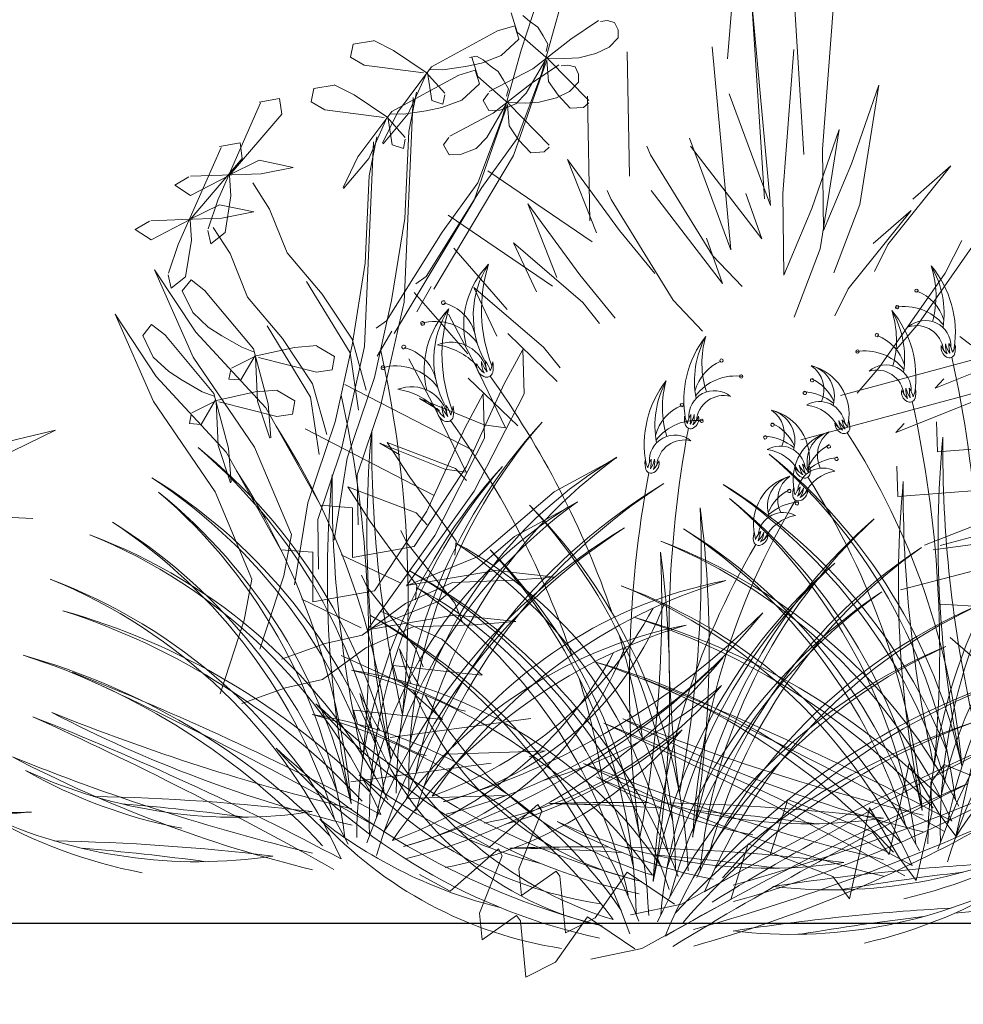
# Model space of a CAD drawing. Units: inches. Extents: x 89 to 490, y -59 to 378.
# Tile 4 of 20: x 300 to 326, y -26 to 1. Entities that reach past the tile are written whole.
import ezdxf

# ---------------------------------------------------------------- set-up
doc = ezdxf.new("R2010")
doc.units = ezdxf.units.IN
doc.header["$MEASUREMENT"] = 0
for name, color, linetype, lineweight in [('A-ANNO-DIMS', 2, 'Continuous', 18), ('L-PLNT', 94, 'Continuous', 18), ('L-PLNT-EDGE', 31, 'Continuous', 25)]:
    doc.layers.add(name, color=color, linetype=linetype, lineweight=lineweight)
doc.layers.add('fl', color=73, linetype='Continuous', lineweight=9, true_color=0xa3d166)
doc.styles.get("Standard").update_dxf_attribs({"font": 'arial.ttf'})
doc.dimstyles.get("Standard").update_dxf_attribs({"dimtxt": 6, "dimasz": 4, "dimexe": 3, "dimexo": 3, "dimgap": 0.09, "dimtad": 0, "dimtih": 1, "dimtoh": 1, "dimdec": 1, "dimzin": 0, "dimdsep": 46, "dimlunit": 3, "dimtxsty": 'Standard', "dimcen": 0.09, "dimadec": 0, "dimazin": 0, "dimtfac": 1, "dimtdec": 1, "dimtofl": 0, "dimtmove": 0, "dimatfit": 3, "dimfxl": 1, "dimtolj": 1, "dimtzin": 0, "dimarcsym": 0})

# ---------------------------------------------------------------- blocks, each defined once
blk = doc.blocks.new('Plantation')
at = {"layer": 'fl'}
for p, q in [((544.751, 40.317), (545.243, 32.557)), ((543.667, 39.099), (544.159, 31.339)), ((543.151, 35.179), (543.425, 38.511)), ((537.49, 35.411), (538.018, 37.033)), ((543.813, 36.723), (544.326, 31.159)), ((537.223, 36.436), (537.387, 35.907)), ((538.054, 34.764), (538.574, 36.629)), ((546.054, 36.651), (545.751, 32.703)), ((537.539, 36.364), (537.724, 36.203)), ((537.724, 36.203), (537.945, 36.043)), ((538.852, 35.714), (539.613, 36.226)), ((539.852, 36.222), (539.671, 36.201)), ((540.053, 36.171), (539.852, 36.222)), ((540.148, 35.972), (540.053, 36.171)), ((535.034, 34.953), (536.847, 35.938)), ((537.317, 36.081), (536.842, 35.939)), ((537.43, 35.711), (537.317, 36.081)), ((537.387, 35.907), (538.239, 35.158)), ((537.945, 36.043), (538.095, 35.809)), ((540.152, 35.754), (540.148, 35.972)), ((533.447, 35.668), (532.891, 35.578)), ((533.453, 35.677), (533.997, 35.404)), ((536.947, 35.264), (537.43, 35.711)), ((537.811, 34.901), (538.852, 35.714)), ((538.095, 35.809), (538.226, 35.574)), ((539.901, 35.494), (540.152, 35.754)), ((532.891, 35.578), (532.818, 35.218)), ((533.997, 35.404), (534.893, 34.802)), ((536.97, 33.546), (537.49, 35.411)), ((538.226, 35.574), (538.175, 35.373)), ((539.54, 35.324), (539.901, 35.494)), ((540.458, 31.956), (540.399, 35.367)), ((542.729, 35.505), (543.242, 29.941)), ((544.97, 35.433), (544.667, 31.485)), ((532.818, 35.218), (533.193, 34.999)), ((536.072, 35.212), (536.272, 35.252)), ((536.14, 35.218), (536.303, 34.689)), ((536.272, 35.252), (536.455, 35.146)), ((536.406, 35.055), (536.947, 35.264)), ((536.455, 35.146), (536.64, 34.985)), ((537.287, 32.524), (538.197, 35.137)), ((537.631, 34.235), (538.179, 35.173)), ((538.197, 35.137), (538.244, 34.555)), ((538.233, 35.192), (538.688, 35.182)), ((538.239, 35.158), (539.347, 34.029)), ((538.688, 35.182), (539.07, 35.207)), ((539.07, 35.207), (539.54, 35.324)), ((533.193, 34.999), (534.817, 34.788)), ((534.104, 33.706), (535.034, 34.953)), ((535.001, 34.884), (535.347, 34.877)), ((535.347, 34.877), (535.969, 34.968)), ((536.234, 34.863), (535.758, 34.721)), ((535.969, 34.968), (536.406, 35.055)), ((536.346, 34.493), (536.234, 34.863)), ((536.616, 34.276), (537.811, 34.901)), ((536.64, 34.985), (536.861, 34.825)), ((536.861, 34.825), (537.011, 34.591)), ((537.768, 34.496), (538.529, 35.008)), ((538.768, 35.004), (538.587, 34.983)), ((538.969, 34.953), (538.768, 35.004)), ((539.064, 34.754), (538.969, 34.953)), ((533.95, 33.735), (535.763, 34.72)), ((534.398, 33.664), (534.897, 34.776)), ((534.893, 34.802), (535.398, 34.236)), ((535.043, 34.034), (534.923, 34.803)), ((536.303, 34.689), (537.155, 33.94)), ((537.011, 34.591), (537.142, 34.356)), ((537.385, 32.991), (538.054, 34.764)), ((538.244, 34.555), (538.505, 34.177)), ((539.068, 34.536), (539.064, 34.754)), ((531.807, 34.36), (531.734, 34)), ((532.363, 34.45), (531.807, 34.36)), ((532.369, 34.459), (532.914, 34.186)), ((535.863, 34.046), (536.346, 34.493)), ((536.727, 33.683), (537.768, 34.496)), ((537.142, 34.356), (537.091, 34.155)), ((538.457, 34.106), (538.817, 34.276)), ((538.817, 34.276), (539.068, 34.536)), ((546.543, 32.293), (547.295, 34.457)), ((547.295, 34.457), (546.775, 31.182)), ((530.309, 33.991), (530.873, 34.089)), ((530.873, 34.089), (530.931, 33.662)), ((532.914, 34.186), (533.809, 33.584)), ((534.528, 34.116), (534.284, 28.508)), ((534.413, 33.182), (534.62, 34.258)), ((535.35, 33.934), (535.043, 34.034)), ((535.322, 33.837), (535.863, 34.046)), ((535.398, 34.187), (535.35, 33.934)), ((536.594, 34.235), (536.452, 34.032)), ((536.452, 34.032), (536.602, 33.762)), ((537.345, 33.938), (537.631, 34.235)), ((537.986, 33.989), (538.457, 34.106)), ((538.505, 34.177), (538.839, 33.819)), ((539.374, 30.738), (539.315, 34.149)), ((544.326, 31.159), (543.192, 34.216)), ((529.72, 32.536), (530.352, 33.967)), ((531.734, 34), (532.109, 33.781)), ((532.109, 33.781), (533.733, 33.57)), ((533.02, 32.488), (533.95, 33.735)), ((534.263, 33.659), (534.885, 33.75)), ((534.885, 33.75), (535.322, 33.837)), ((536.203, 31.306), (537.114, 33.919)), ((536.547, 33.017), (537.095, 33.955)), ((536.602, 33.762), (536.912, 33.767)), ((536.912, 33.767), (537.345, 33.938)), ((537.114, 33.919), (537.16, 33.337)), ((537.149, 33.974), (537.604, 33.964)), ((537.155, 33.94), (538.263, 32.811)), ((537.604, 33.964), (537.986, 33.989)), ((538.839, 33.819), (539.202, 33.843)), ((539.202, 33.843), (539.346, 33.973)), ((530.931, 33.662), (529.502, 31.99)), ((533.315, 32.446), (533.813, 33.558)), ((533.695, 32.866), (534.104, 33.706)), ((533.709, 32.842), (534.398, 33.664)), ((533.809, 33.584), (534.314, 33.018)), ((533.959, 32.816), (533.839, 33.585)), ((533.917, 33.666), (534.263, 33.659)), ((535.533, 33.058), (536.727, 33.683)), ((536.301, 31.773), (536.97, 33.546)), ((537.16, 33.337), (537.421, 32.959)), ((545.459, 31.075), (546.211, 33.239)), ((546.211, 33.239), (545.691, 29.964)), ((533.33, 31.964), (533.536, 33.04)), ((534.315, 32.969), (534.266, 32.716)), ((534.3, 30.796), (534.413, 33.182)), ((535.51, 33.017), (535.368, 32.814)), ((536.261, 32.72), (536.547, 33.017)), ((536.41, 31.646), (537.385, 32.991)), ((537.421, 32.959), (537.755, 32.601)), ((543.242, 29.941), (542.108, 32.998)), ((528.636, 31.318), (529.268, 32.749)), ((529.225, 32.773), (529.789, 32.871)), ((529.789, 32.871), (529.847, 32.444)), ((533.444, 32.898), (533.2, 27.29)), ((534.266, 32.716), (533.959, 32.816)), ((535.368, 32.814), (535.518, 32.544)), ((535.828, 32.549), (536.261, 32.72)), ((538.119, 32.625), (538.262, 32.755)), ((540.935, 32.782), (541.041, 32.543)), ((542.136, 32.784), (544.093, 30.239)), ((545.751, 32.703), (545.778, 30.468)), ((529.847, 32.444), (528.418, 30.772)), ((529.179, 31.302), (529.72, 32.536)), ((530.312, 32.394), (529.465, 31.976)), ((531.245, 32.196), (530.312, 32.394)), ((532.611, 31.648), (533.02, 32.488)), ((532.625, 31.624), (533.315, 32.446)), ((535.097, 28.864), (537.287, 32.524)), ((535.518, 32.544), (535.828, 32.549)), ((537.755, 32.601), (538.119, 32.625)), ((539.558, 30.402), (538.76, 32.416)), ((538.76, 32.416), (540.188, 30.472)), ((541.041, 32.543), (542.739, 29.781)), ((530.369, 32.023), (531.239, 32.198)), ((545.778, 30.468), (546.543, 32.293)), ((549.267, 32.24), (547.541, 30.09)), ((548.228, 31.329), (549.267, 32.24)), ((528.385, 31.945), (527.999, 31.712)), ((528.427, 31.957), (529.301, 31.987)), ((528.431, 31.43), (529.49, 31.977)), ((529.301, 31.987), (530.369, 32.023)), ((529.537, 31.424), (529.502, 31.977)), ((533.216, 29.578), (533.33, 31.964)), ((539.439, 30.158), (536.579, 32.105)), ((527.999, 31.712), (528.431, 31.43)), ((530.135, 31.772), (530.597, 31.058)), ((534.889, 29.212), (536.41, 31.646)), ((535.326, 30.428), (536.301, 31.773)), ((528.095, 30.084), (528.636, 31.318)), ((529.379, 30.415), (529.537, 31.424)), ((534.013, 27.646), (536.203, 31.306)), ((539.852, 31.564), (539.957, 31.324)), ((539.957, 31.324), (541.655, 28.563)), ((541.053, 31.566), (543.009, 29.021)), ((544.093, 30.239), (543.655, 31.48)), ((544.667, 31.485), (544.695, 29.25)), ((529.228, 31.176), (528.381, 30.758)), ((528.914, 30.515), (529.179, 31.302)), ((530.161, 30.978), (529.228, 31.176)), ((530.597, 31.058), (531.075, 29.859)), ((538.474, 29.184), (537.677, 31.198)), ((537.677, 31.198), (539.104, 29.254)), ((544.695, 29.25), (545.459, 31.075)), ((546.775, 31.182), (546.061, 29.311)), ((527.343, 30.739), (528.217, 30.769)), ((528.217, 30.769), (529.286, 30.805)), ((529.286, 30.805), (530.155, 30.98)), ((533.94, 28.547), (534.3, 30.796)), ((538.355, 28.94), (535.495, 30.887)), ((548.183, 31.022), (546.458, 28.872)), ((547.144, 30.111), (548.183, 31.022)), ((527.301, 30.727), (526.915, 30.494)), ((527.348, 30.212), (528.406, 30.759)), ((528.453, 30.206), (528.419, 30.759)), ((529.051, 30.554), (529.513, 29.84)), ((550.2, 30.521), (548.393, 27.932)), ((526.915, 30.494), (527.348, 30.212)), ((528.901, 30.47), (528.982, 30.107)), ((528.982, 30.107), (529.379, 30.415)), ((533.805, 27.994), (535.326, 30.428)), ((540.188, 30.472), (541.152, 29.289)), ((543.009, 29.021), (542.572, 30.262)), ((527.83, 29.297), (528.095, 30.084)), ((528.295, 29.197), (528.453, 30.206)), ((535.646, 29.986), (537.112, 28.305)), ((537.912, 28.79), (537.283, 30.13)), ((537.283, 30.13), (539.186, 28.493)), ((545.691, 29.964), (544.977, 28.093)), ((547.541, 30.09), (547.178, 29.349)), ((549.572, 30.194), (549.117, 29.303)), ((529.513, 29.84), (529.991, 28.641)), ((531.075, 29.859), (532.038, 28.726)), ((542.739, 29.781), (543.546, 28.933)), ((532.856, 27.329), (533.216, 29.578)), ((528.499, 27.001), (527.445, 29.395)), ((527.445, 29.395), (528.573, 27.684)), ((527.817, 29.252), (527.898, 28.889)), ((527.898, 28.889), (528.295, 29.197)), ((534.604, 29.008), (534.889, 29.212)), ((539.104, 29.254), (540.068, 28.071)), ((549.117, 29.303), (547.309, 26.714)), ((528.205, 28.812), (528.446, 29.115)), ((528.446, 29.115), (528.836, 28.808)), ((531.611, 29.076), (532.806, 27.116)), ((534.63, 28.241), (535.028, 28.931)), ((536.828, 27.572), (536.199, 28.912)), ((536.199, 28.912), (538.102, 27.275)), ((528.49, 28.219), (528.205, 28.812)), ((530.154, 27.225), (528.831, 28.809)), ((529.991, 28.641), (530.954, 27.508)), ((532.038, 28.726), (532.857, 27.49)), ((534.563, 28.768), (536.028, 27.087)), ((546.458, 28.872), (546.094, 28.131)), ((533.477, 26.441), (533.94, 28.547)), ((534.284, 28.508), (533.65, 25.695)), ((539.186, 28.493), (539.643, 27.925)), ((541.655, 28.563), (542.462, 27.715)), ((527.415, 25.783), (526.361, 28.177)), ((526.361, 28.177), (527.489, 26.466)), ((528.916, 27.825), (528.49, 28.219)), ((536.23, 26.788), (535.502, 28.173)), ((527.121, 27.594), (527.363, 27.897)), ((527.363, 27.897), (527.753, 27.59)), ((529.289, 27.583), (528.916, 27.825)), ((530.527, 27.858), (531.722, 25.898)), ((533.521, 27.79), (533.805, 27.994)), ((548.393, 27.932), (547.785, 27.231)), ((527.406, 27.001), (527.121, 27.594)), ((529.07, 26.007), (527.747, 27.591)), ((528.573, 27.684), (530.491, 25.61)), ((529.835, 27.269), (529.289, 27.583)), ((533.546, 27.023), (533.944, 27.713)), ((537.124, 27.645), (538.482, 26.33)), ((552.203, 27.553), (546.246, 25.952)), ((548.842, 26.149), (552.295, 27.53)), ((549.516, 27.567), (549.816, 27.334)), ((530.158, 27.149), (529.835, 27.269)), ((531.283, 27.262), (530.229, 27.033)), ((530.954, 27.508), (531.774, 26.272)), ((531.889, 27.315), (531.283, 27.262)), ((531.892, 27.304), (532.376, 27.016)), ((532.393, 25.223), (532.856, 27.329)), ((533.2, 27.29), (532.566, 24.477)), ((532.857, 27.49), (533.245, 26.093)), ((538.102, 27.275), (538.559, 26.707)), ((527.832, 26.607), (527.406, 27.001)), ((530.187, 24.53), (528.499, 27.001)), ((530.229, 27.033), (529.55, 26.693)), ((529.807, 26.374), (530.201, 27.045)), ((530.558, 25.723), (530.154, 27.225)), ((530.269, 25.793), (530.215, 27.01)), ((531.881, 26.589), (530.294, 26.991)), ((532.376, 27.016), (532.311, 26.654)), ((532.806, 27.116), (533.038, 25.548)), ((537.031, 26.271), (537.534, 27.212)), ((537.534, 27.212), (537.575, 25.998)), ((535.146, 25.57), (534.418, 26.955)), ((537.067, 25.066), (536.23, 26.788)), ((527.489, 26.466), (529.407, 24.392)), ((528.205, 26.365), (527.832, 26.607)), ((529.532, 26.647), (529.484, 26.394)), ((532.311, 26.654), (531.881, 26.589)), ((547.309, 26.714), (546.701, 26.013)), ((528.751, 26.051), (528.205, 26.365)), ((529.484, 26.394), (529.807, 26.374)), ((531.774, 26.272), (532.162, 24.875)), ((536.192, 24.428), (532.66, 26.252)), ((532.726, 24.228), (533.477, 26.441)), ((535.99, 23.999), (537.031, 26.271)), ((536.041, 26.427), (537.398, 25.112)), ((551.119, 26.335), (545.162, 24.734)), ((547.759, 24.931), (551.212, 26.312)), ((549.077, 26.4), (548.842, 26.149)), ((529.074, 25.931), (528.751, 26.051)), ((529.474, 24.505), (529.07, 26.007)), ((530.199, 26.044), (529.145, 25.815)), ((530.806, 26.097), (530.199, 26.044)), ((530.808, 26.086), (531.292, 25.798)), ((535.947, 25.053), (536.45, 25.994)), ((537.575, 25.998), (536.208, 23.326)), ((536.45, 25.994), (536.491, 24.78)), ((529.104, 23.312), (527.415, 25.783)), ((529.145, 25.815), (528.466, 25.475)), ((528.723, 25.156), (529.117, 25.827)), ((529.185, 24.575), (529.132, 25.792)), ((530.797, 25.371), (529.21, 25.773)), ((530.607, 24.774), (530.269, 25.793)), ((530.628, 24.791), (530.558, 25.723)), ((531.292, 25.798), (531.227, 25.436)), ((531.722, 25.898), (531.954, 24.33)), ((533.65, 25.695), (533.001, 23.77)), ((535.252, 25.539), (534.706, 25.861)), ((534.706, 25.861), (536.481, 25.144)), ((528.448, 25.429), (528.4, 25.176)), ((530.491, 25.61), (531.992, 22.939)), ((531.227, 25.436), (530.797, 25.371)), ((535.983, 23.848), (535.146, 25.57)), ((528.4, 25.176), (528.723, 25.156)), ((531.642, 23.01), (532.393, 25.223)), ((536.481, 25.144), (537.067, 25.066)), ((547.993, 25.182), (547.759, 24.931)), ((548.874, 25.226), (548.902, 24.401)), ((524.733, 24.997), (522.589, 23.962)), ((523.242, 24.639), (524.733, 24.997)), ((535.108, 23.21), (531.576, 25.034)), ((534.907, 22.781), (535.947, 25.053)), ((529.523, 23.556), (529.185, 24.575)), ((534.168, 24.321), (533.622, 24.643)), ((533.622, 24.643), (535.397, 23.926)), ((534.439, 23.713), (533.823, 24.664)), ((533.823, 24.664), (535.695, 23.95)), ((536.491, 24.78), (535.124, 22.108)), ((548.902, 24.401), (552.345, 24.664)), ((529.407, 24.392), (530.908, 21.721)), ((529.544, 23.573), (529.474, 24.505)), ((531.193, 22.134), (530.187, 24.53)), ((532.566, 24.477), (531.917, 22.552)), ((532.365, 21.98), (532.726, 24.228)), ((538.396, 23.303), (540.114, 24.237)), ((533.001, 23.77), (533.025, 22.404)), ((534.558, 21.811), (535.99, 23.999)), ((535.397, 23.926), (535.983, 23.848)), ((535.695, 23.95), (535.998, 23.62)), ((547.79, 24.008), (547.818, 23.183)), ((535.714, 21.958), (534.439, 23.713)), ((530.109, 20.916), (529.104, 23.312)), ((533.355, 22.495), (532.739, 23.446)), ((532.739, 23.446), (534.611, 22.732)), ((536.208, 23.326), (534.352, 20.735)), ((536.318, 21.531), (538.396, 23.303)), ((547.818, 23.183), (551.261, 23.446)), ((531.281, 20.762), (531.642, 23.01)), ((531.992, 22.939), (532.869, 22.872)), ((537.312, 22.085), (539.031, 23.019)), ((520.615, 22.763), (524.11, 22.574)), ((532.869, 22.872), (532.867, 21.511)), ((533.474, 20.593), (534.907, 22.781)), ((534.611, 22.732), (534.914, 22.402)), ((550.991, 22.805), (548.544, 21.846)), ((531.917, 22.552), (531.941, 21.186)), ((534.63, 20.74), (533.355, 22.495)), ((552.039, 22.642), (548.978, 21.84)), ((530.988, 21.009), (531.193, 22.134)), ((534.355, 21.911), (534.197, 22.246)), ((535.124, 22.108), (533.268, 19.517)), ((535.675, 20.255), (534.355, 21.911)), ((535.234, 20.313), (537.312, 22.085)), ((535.679, 21.568), (535.714, 21.958)), ((548.789, 21.719), (551.609, 22.101)), ((530.908, 21.721), (531.785, 21.654)), ((531.785, 21.654), (531.783, 20.293)), ((532.867, 21.511), (534.558, 21.811)), ((532.562, 21.58), (534.191, 20.801)), ((534.352, 20.735), (536.318, 21.531)), ((550.955, 21.424), (547.894, 20.622)), ((536.74, 21.145), (534.353, 20.74)), ((536.719, 21.156), (538.427, 20.971)), ((529.904, 19.791), (530.109, 20.916)), ((530.328, 18.993), (530.988, 21.009)), ((533.271, 20.693), (533.113, 21.028)), ((535.613, 20.826), (534.32, 20.248)), ((537.263, 20.883), (535.613, 20.826)), ((538.427, 20.971), (537.263, 20.883)), ((531.783, 20.293), (533.474, 20.593)), ((534.591, 19.037), (533.271, 20.693)), ((534.595, 20.35), (534.63, 20.74)), ((531.478, 20.362), (533.107, 19.583)), ((534.32, 20.248), (533.134, 19.381)), ((533.268, 19.517), (535.234, 20.313)), ((535.887, 19.727), (535.675, 20.255)), ((535.32, 19.271), (533.641, 20.04)), ((548.981, 20.225), (552.476, 20.037)), ((529.244, 17.775), (529.904, 19.791)), ((535.657, 19.927), (533.269, 19.522)), ((535.636, 19.938), (537.343, 19.753)), ((537.343, 19.753), (536.18, 19.665)), ((534.529, 19.608), (533.236, 19.03)), ((536.18, 19.665), (534.529, 19.608)), ((533.134, 19.381), (532.121, 19.152)), ((536.423, 18.287), (535.32, 19.271)), ((549.247, 19.315), (551.779, 17.113)), ((532.121, 19.152), (530.92, 18.722)), ((533.236, 19.03), (532.05, 18.163)), ((534.804, 18.509), (534.591, 19.037)), ((534.236, 18.053), (532.557, 18.822)), ((534.094, 18.159), (533.983, 18.544)), ((533.983, 18.544), (535.691, 18.36)), ((535.691, 18.36), (536.423, 18.287)), ((532.05, 18.163), (531.037, 17.934)), ((535.774, 17.342), (534.094, 18.159)), ((531.037, 17.934), (529.836, 17.504)), ((535.339, 17.069), (534.236, 18.053)), ((533.01, 16.941), (532.899, 17.326)), ((532.899, 17.326), (534.607, 17.142)), ((535.97, 17.3), (535.774, 17.342)), ((533.906, 16.575), (537.756, 17.091)), ((534.607, 17.142), (535.339, 17.069)), ((534.69, 16.124), (533.01, 16.941)), ((538.146, 16.207), (537.175, 16.174)), ((537.714, 16.047), (538.146, 16.207)), ((534.886, 16.082), (534.69, 16.124)), ((537.175, 16.174), (535.476, 16.116)), ((532.822, 15.357), (536.672, 15.873)), ((548.124, 15.867), (547.577, 13.369)), ((548.949, 14.485), (548.124, 15.867)), ((549.09, 15.837), (548.718, 15.338)), ((550.076, 15.433), (549.09, 15.837)), ((549.83, 15.731), (549.407, 13.869)), ((548.718, 15.338), (548.746, 14.513)), ((536.091, 14.956), (534.392, 14.898)), ((537.063, 14.989), (536.091, 14.956)), ((536.631, 14.829), (537.063, 14.989)), ((544.803, 14.879), (544.32, 13.355)), ((547.118, 13.985), (544.803, 14.879)), ((537.953, 14.742), (536.632, 13.579)), ((538.057, 14.551), (537.953, 14.742)), ((547.04, 14.649), (546.493, 12.151)), ((547.865, 13.267), (547.04, 14.649)), ((537.43, 12.974), (538.057, 14.551)), ((548.746, 14.513), (548.323, 12.651)), ((549.407, 13.869), (548.949, 14.485)), ((536.632, 13.579), (535.79, 14.036)), ((547.577, 13.369), (547.118, 13.985)), ((536.869, 13.524), (535.548, 12.361)), ((536.973, 13.333), (536.869, 13.524)), ((543.719, 13.661), (543.236, 12.137)), ((546.034, 12.767), (543.719, 13.661)), ((536.346, 11.756), (536.973, 13.333)), ((544.32, 13.355), (541.887, 12.008)), ((548.323, 12.651), (547.865, 13.267)), ((537.504, 12.248), (537.43, 12.974)), ((535.548, 12.361), (534.706, 12.818)), ((538.453, 12.912), (537.504, 12.248)), ((538.555, 12.77), (538.453, 12.912)), ((538.705, 11.219), (538.555, 12.77)), ((540.399, 12.881), (539.518, 11.636)), ((541.693, 12.002), (540.399, 12.881)), ((546.493, 12.151), (546.034, 12.767)), ((541.887, 12.008), (540.487, 11.717)), ((543.236, 12.137), (540.803, 10.79)), ((536.42, 11.03), (536.346, 11.756)), ((537.369, 11.694), (536.42, 11.03)), ((537.471, 11.552), (537.369, 11.694)), ((539.315, 11.663), (538.434, 10.418)), ((539.518, 11.636), (538.705, 11.219)), ((540.609, 10.784), (539.315, 11.663)), ((537.622, 10.001), (537.471, 11.552)), ((540.803, 10.79), (539.403, 10.499)), ((538.434, 10.418), (537.622, 10.001))]:
    blk.add_line(p, q, dxfattribs=at)
for centre, radius, start, end in [((538.293, 27.882), 2.375, 135.5632, 193.7293), ((538.781, 28.132), 2.601, 147.096, 209.2874), ((540.633, 28.287), 4.227, 162.6858, 201.1197), ((546.541, 27.672), 2.854, 351.4134, 39.8275), ((546.256, 28.682), 2.608, 344.3064, 18.279), ((546.485, 28.192), 2.6, 351.5096, 30.1949), ((548.325, 28.821), 0.0459, 7.5892, 187.5892), ((548.325, 28.821), 0.0459, 187.5892, 7.5892), ((547.89, 27.65), 1.243, 16.8512, 68.8014), ((535.359, 28.494), 0.053, 11.802, 191.802), ((535.359, 28.494), 0.053, 191.802, 11.802), ((535.098, 27.351), 1.163, 13.7128, 76.1437), ((547.799, 28.369), 0.0459, 7.5892, 187.5892), ((547.997, 27.001), 1.386, 39.5069, 100.1323), ((547.799, 28.369), 0.0459, 187.5892, 7.5892), ((537.21, 26.664), 2.375, 135.5632, 193.7293), ((537.697, 26.914), 2.601, 147.096, 209.2874), ((539.549, 27.069), 4.227, 162.6858, 201.1197), ((545.457, 26.454), 2.854, 351.4134, 39.8275), ((545.172, 27.464), 2.608, 344.3064, 18.279), ((545.401, 26.974), 2.6, 351.5096, 30.1949), ((534.791, 27.927), 0.053, 11.802, 191.802), ((535.138, 26.561), 1.416, 35.6636, 106.404), ((534.791, 27.927), 0.053, 191.802, 11.802), ((548.57, 27.303), 0.701, 357.4175, 130.8703), ((548.32, 27.109), 0.754, 6.9832, 106.1055), ((544.805, 25.819), 2.854, 142.1725, 190.5866), ((544.843, 26.34), 2.6, 151.8051, 190.4904), ((545.055, 26.838), 2.608, 163.721, 197.6936), ((547.241, 27.603), 0.0459, 7.5892, 187.5892), ((547.241, 27.603), 0.0459, 187.5892, 7.5892), ((546.806, 26.432), 1.243, 16.8512, 68.8014), ((534.275, 27.276), 0.053, 11.802, 191.802), ((534.275, 27.276), 0.053, 191.802, 11.802), ((534.014, 26.132), 1.163, 13.7128, 76.1437), ((535.571, 26.397), 1.01, 11.1862, 111.7493), ((534.913, 25.471), 1.886, 44.0209, 81.3627), ((549.289, 27.258), 0.289, 168.1654, 242.3938), ((549.56, 27.536), 0.596, 201.5294, 228.9216), ((549.687, 27.312), 0.565, 174.5103, 203.5444), ((549.838, 27.532), 0.733, 193.0983, 215.538), ((550.524, 27.366), 1.308, 179.8013, 191.4565), ((548.639, 26.985), 0.694, 12.1333, 33.7421), ((548.367, 27.577), 1.049, 334.86, 346.6738), ((548.799, 27.25), 0.595, 343.9406, 8.2206), ((502.903, 20.338), 31.492, 354.2791, 12.5427), ((546.715, 27.151), 0.0459, 7.5892, 187.5892), ((546.914, 25.783), 1.386, 39.5069, 100.1323), ((546.715, 27.151), 0.0459, 187.5892, 7.5892), ((549.228, 27.134), 0.151, 241.146, 341.1111), ((518.556, 20.16), 31.492, 354.2791, 12.5427), ((533.707, 26.709), 0.053, 11.802, 191.802), ((534.055, 25.343), 1.416, 35.6636, 106.404), ((533.707, 26.709), 0.053, 191.802, 11.802), ((536.603, 26.772), 0.334, 172.3781, 246.6066), ((536.893, 27.116), 0.689, 205.7422, 233.1344), ((537.058, 26.869), 0.654, 178.723, 207.7572), ((537.214, 27.135), 0.848, 197.3111, 219.7508), ((535.876, 26.402), 0.803, 16.3461, 37.9549), ((538.019, 27.002), 1.513, 184.0141, 195.6693), ((535.514, 27.061), 1.213, 339.0728, 350.8866), ((536.04, 26.721), 0.688, 348.1534, 12.4334), ((543.458, 25.75), 1.243, 113.1986, 165.1488), ((542.982, 26.905), 0.0459, 354.4108, 174.4108), ((542.982, 26.905), 0.0459, 174.4108, 354.4108), ((545.216, 25.932), 0.863, 342.816, 75.0201), ((544.998, 26.106), 0.793, 335.7976, 56.2278), ((545.111, 25.437), 1.368, 349.633, 76.1366), ((547.486, 26.085), 0.701, 357.4175, 130.8703), ((536.544, 26.624), 0.175, 245.3588, 345.3239), ((516.603, 12.04), 24.696, 18.7875, 35.7756), ((543.373, 25.098), 1.386, 81.8677, 142.4931), ((543.523, 26.471), 0.0459, 354.4108, 174.4108), ((543.523, 26.471), 0.0459, 174.4108, 354.4108), ((547.237, 25.891), 0.754, 6.9832, 106.1055), ((534.487, 25.179), 1.01, 11.1862, 111.7493), ((543.721, 24.601), 2.854, 142.1725, 190.5866), ((543.759, 25.122), 2.6, 151.8051, 190.4904), ((543.971, 25.62), 2.608, 163.721, 197.6936), ((545.466, 26.365), 0.0459, 19.649, 199.649), ((545.466, 26.365), 0.0459, 199.649, 19.649), ((544.931, 25.279), 1.243, 24.0842, 65.3008), ((501.819, 19.12), 31.492, 354.2791, 12.5427), ((533.829, 24.253), 1.886, 44.0209, 81.3627), ((542.79, 25.379), 0.701, 51.1297, 184.5825), ((543.046, 25.194), 0.754, 75.8945, 175.0168), ((545.267, 26.018), 0.0459, 19.649, 199.649), ((545.267, 26.018), 0.0459, 199.649, 19.649), ((545.172, 24.667), 1.386, 50.416, 87.3549), ((548.205, 26.04), 0.289, 168.1654, 242.3938), ((548.477, 26.318), 0.596, 201.5294, 228.9216), ((548.603, 26.094), 0.565, 174.5103, 203.5444), ((548.754, 26.314), 0.733, 193.0983, 215.538), ((549.44, 26.148), 1.308, 179.8013, 191.4565), ((547.555, 25.767), 0.694, 12.1333, 33.7421), ((547.284, 26.359), 1.049, 334.86, 346.6738), ((547.716, 26.032), 0.595, 343.9406, 8.2206), ((535.974, 25.65), 0.654, 178.723, 207.7572), ((536.13, 25.917), 0.848, 197.3111, 219.7508), ((534.793, 25.184), 0.803, 16.3461, 37.9549), ((536.935, 25.784), 1.513, 184.0141, 195.6693), ((534.43, 25.843), 1.213, 339.0728, 350.8866), ((534.956, 25.503), 0.688, 348.1534, 12.4334), ((542.374, 24.532), 1.243, 113.1986, 165.1488), ((541.898, 25.687), 0.0459, 354.4108, 174.4108), ((541.898, 25.687), 0.0459, 174.4108, 354.4108), ((545.674, 25.086), 0.696, 9.2042, 120.225), ((545.159, 24.545), 1.154, 27.9293, 81.8071), ((548.144, 25.916), 0.151, 241.146, 341.1111), ((517.472, 18.942), 31.492, 354.2791, 12.5427), ((535.52, 25.554), 0.334, 172.3781, 246.6066), ((535.809, 25.898), 0.689, 205.7422, 233.1344), ((542.563, 25.318), 0.595, 173.7794, 198.0594), ((542.983, 25.66), 1.049, 195.3262, 207.14), ((542.733, 25.059), 0.694, 148.2579, 169.8667), ((540.835, 25.374), 1.308, 350.5435, 2.1987), ((541.515, 25.564), 0.733, 326.462, 348.9017), ((541.674, 25.349), 0.565, 338.4556, 7.4897), ((541.792, 25.577), 0.596, 313.0784, 340.4706), ((542.073, 25.309), 0.289, 299.6062, 13.8346), ((544.132, 24.714), 0.863, 342.816, 75.0201), ((543.914, 24.888), 0.793, 335.7976, 56.2278), ((544.027, 24.219), 1.368, 349.633, 76.1366), ((513.782, 14.158), 20.216, 5.151, 32.7872), ((549.271, 14.948), 15.201, 137.4916, 179.6099), ((549.333, 15.438), 14.921, 139.0392, 181.297), ((535.46, 25.406), 0.175, 245.3588, 345.3239), ((515.52, 10.822), 24.696, 18.7875, 35.7756), ((542.289, 23.88), 1.386, 81.8677, 142.4931), ((542.138, 25.187), 0.151, 200.8889, 300.854), ((542.439, 25.253), 0.0459, 174.4108, 354.4108), ((542.439, 25.253), 0.0459, 354.4108, 174.4108), ((544.382, 25.147), 0.0459, 19.649, 199.649), ((544.382, 25.147), 0.0459, 199.649, 19.649), ((543.847, 24.061), 1.243, 24.0842, 65.3008), ((546.381, 25.187), 0.289, 180.2252, 254.4537), ((546.589, 25.516), 0.596, 213.5892, 240.9815), ((546.759, 25.324), 0.565, 186.5701, 215.6042), ((546.861, 25.571), 0.733, 205.1582, 227.5978), ((545.802, 24.785), 0.694, 24.1932, 45.802), ((547.567, 25.551), 1.308, 191.8611, 203.5164), ((545.414, 25.307), 1.049, 346.9198, 358.7337), ((545.904, 25.077), 0.595, 356.0005, 20.2804), ((563.159, 22.183), 29.894, 174.6174, 191.9895), ((567.384, 24.718), 33.989, 179.5471, 192.7817), ((541.706, 24.161), 0.701, 51.1297, 184.5825), ((573.035, 19.288), 31.492, 169.4573, 187.7209), ((544.183, 24.8), 0.0459, 19.649, 199.649), ((544.088, 23.449), 1.386, 50.416, 87.3549), ((546.312, 23.635), 1.368, 105.8634, 192.367), ((546.19, 24.126), 0.863, 106.9799, 199.184), ((546.402, 24.308), 0.793, 125.7722, 206.2024), ((546.348, 25.054), 0.151, 253.2058, 353.1709), ((529.435, 13.979), 20.216, 5.151, 32.7872), ((541.962, 23.976), 0.754, 75.8945, 175.0168), ((544.183, 24.8), 0.0459, 199.649, 19.649), ((544.59, 23.867), 0.696, 9.2042, 120.225), ((546.497, 23.483), 1.243, 116.6992, 157.9158), ((545.925, 24.55), 0.0459, 162.351, 342.351), ((545.925, 24.55), 0.0459, 342.351, 162.351), ((578.812, 22.005), 29.894, 174.6174, 191.9895), ((583.037, 24.54), 33.989, 179.5471, 192.7817), ((518.937, 13.181), 14.921, 7.1968, 49.4547), ((519.071, 12.705), 15.201, 12.4122, 51.0023), ((544.075, 23.327), 1.154, 27.9293, 81.8071), ((534.591, 13.003), 14.921, 7.1968, 49.4547), ((534.724, 12.527), 15.201, 12.4122, 51.0023), ((546.191, 13.886), 12.017, 120.3536, 167.8423), ((548.22, 13.014), 13.856, 125.7805, 169.1581), ((541.479, 24.1), 0.595, 173.7794, 198.0594), ((541.899, 24.442), 1.049, 195.3262, 207.14), ((541.649, 23.841), 0.694, 148.2579, 169.8667), ((539.751, 24.156), 1.308, 350.5435, 2.1987), ((540.431, 24.346), 0.733, 326.462, 348.9017), ((540.59, 24.131), 0.565, 338.4556, 7.4897), ((540.708, 24.359), 0.596, 313.0784, 340.4706), ((540.989, 24.091), 0.289, 299.6062, 13.8346), ((545.675, 24.106), 0.565, 186.5701, 215.6042), ((545.778, 24.353), 0.733, 205.1582, 227.5978), ((544.719, 23.567), 0.694, 24.1932, 45.802), ((546.483, 24.333), 1.308, 191.8611, 203.5164), ((544.33, 24.089), 1.049, 346.9198, 358.7337), ((546.278, 22.863), 1.386, 94.6451, 131.584), ((544.821, 23.859), 0.595, 356.0005, 20.2804), ((546.136, 24.21), 0.0459, 162.351, 342.351), ((546.136, 24.21), 0.0459, 342.351, 162.351), ((512.698, 12.94), 20.216, 5.151, 32.7872), ((562.075, 20.965), 29.894, 174.6174, 191.9895), ((566.3, 23.5), 33.989, 179.5471, 192.7817), ((548.187, 13.73), 15.201, 137.4916, 179.6099), ((548.249, 14.22), 14.921, 139.0392, 181.297), ((571.951, 18.07), 31.492, 169.4573, 187.7209), ((541.055, 23.969), 0.151, 200.8889, 300.854), ((545.298, 23.969), 0.289, 180.2252, 254.4537), ((545.505, 24.298), 0.596, 213.5892, 240.9815), ((545.762, 23.264), 0.696, 61.775, 172.7958), ((545.264, 23.836), 0.151, 253.2058, 353.1709), ((546.296, 22.742), 1.154, 100.1929, 154.0707), ((563.84, 13.552), 15.201, 137.4916, 179.6099), ((563.902, 14.042), 14.921, 139.0392, 181.297), ((519.189, 11.215), 14.921, 16.8321, 56.7339), ((519.381, 10.76), 15.201, 21.5651, 58.2814), ((550.014, 9.293), 16.642, 121.1471, 160.292), ((550.148, 9.85), 16.239, 122.567, 163.1344), ((534.842, 11.037), 14.921, 16.8321, 56.7339), ((535.034, 10.582), 15.201, 21.5651, 58.2814), ((545.228, 22.417), 1.368, 105.8634, 192.367), ((545.107, 22.908), 0.863, 106.9799, 199.184), ((545.318, 23.09), 0.793, 125.7722, 206.2024), ((528.351, 12.761), 20.216, 5.151, 32.7872), ((577.728, 20.787), 29.894, 174.6174, 191.9895), ((581.953, 23.322), 33.989, 179.5471, 192.7817), ((517.854, 11.963), 14.921, 7.1968, 49.4547), ((517.987, 11.487), 15.201, 12.4122, 51.0023), ((545.413, 22.265), 1.243, 116.6992, 157.9158), ((544.841, 23.332), 0.0459, 162.351, 342.351), ((544.841, 23.332), 0.0459, 342.351, 162.351), ((545.532, 23.248), 0.595, 161.7196, 185.9995), ((546.014, 23.494), 1.049, 183.2663, 195.0802), ((545.644, 22.959), 0.694, 136.198, 157.8068), ((543.854, 23.664), 1.308, 338.4836, 350.1389), ((544.558, 23.708), 0.733, 314.4022, 336.8418), ((545.051, 23.341), 0.289, 287.5463, 1.7748), ((544.669, 23.464), 0.565, 326.3958, 355.4299), ((544.832, 23.663), 0.596, 301.0185, 328.4108), ((545.107, 12.667), 12.017, 120.3536, 167.8423), ((547.136, 11.796), 13.856, 125.7805, 169.1581), ((526.805, 12.771), 14.921, 0.703, 42.9608), ((526.883, 12.283), 15.201, 2.3901, 44.5084), ((562.379, 12.732), 20.216, 149.2128, 176.849), ((533.507, 11.785), 14.921, 7.1968, 49.4547), ((533.64, 11.309), 15.201, 12.4122, 51.0023), ((545.194, 21.645), 1.386, 94.6451, 131.584), ((545.089, 23.209), 0.151, 188.8291, 288.7942), ((545.052, 22.992), 0.0459, 162.351, 342.351), ((545.052, 22.992), 0.0459, 342.351, 162.351), ((508.441, 21.415), 33.989, 349.2183, 2.4529), ((512.752, 19.029), 29.894, 350.0105, 7.3826), ((544.678, 22.046), 0.696, 61.775, 172.7958), ((560.76, 12.489), 12.017, 120.3536, 167.8423), ((562.789, 11.618), 13.856, 125.7805, 169.1581), ((518.105, 9.997), 14.921, 16.8321, 56.7339), ((518.297, 9.542), 15.201, 21.5651, 58.2814), ((557.143, 11.096), 15.201, 130.9977, 169.5878), ((557.26, 11.576), 14.921, 132.5453, 174.8032), ((545.212, 21.524), 1.154, 100.1929, 154.0707), ((520.326, 7.9), 15.201, 27.2807, 69.4256), ((520.05, 8.309), 14.921, 24.3637, 67.878), ((548.931, 8.075), 16.642, 121.1471, 160.292), ((549.064, 8.632), 16.239, 122.567, 163.1344), ((533.758, 9.819), 14.921, 16.8321, 56.7339), ((533.951, 9.364), 15.201, 21.5651, 58.2814), ((544.448, 22.03), 0.595, 161.7196, 185.9995), ((544.93, 22.276), 1.049, 183.2663, 195.0802), ((544.56, 21.741), 0.694, 136.198, 157.8068), ((542.77, 22.446), 1.308, 338.4836, 350.1389), ((543.474, 22.49), 0.733, 314.4022, 336.8418), ((543.967, 22.123), 0.289, 287.5463, 1.7748), ((543.585, 22.246), 0.565, 326.3958, 355.4299), ((543.748, 22.445), 0.596, 301.0185, 328.4108), ((564.584, 7.897), 16.642, 121.1471, 160.292), ((564.717, 8.454), 16.239, 122.567, 163.1344), ((528.001, 10.387), 13.856, 12.8419, 56.2195), ((529.999, 11.329), 12.017, 14.1577, 61.6464), ((561.295, 11.514), 20.216, 149.2128, 176.849), ((535.98, 7.721), 15.201, 27.2807, 69.4256), ((535.703, 8.13), 14.921, 24.3637, 67.878), ((544.006, 21.991), 0.151, 188.8291, 288.7942), ((525.721, 11.553), 14.921, 0.703, 42.9608), ((525.8, 11.065), 15.201, 2.3901, 44.5084), ((507.357, 20.197), 33.989, 349.2183, 2.4529), ((511.668, 17.811), 29.894, 350.0105, 7.3826), ((556.901, 9.141), 15.201, 123.7186, 160.4349), ((557.078, 9.602), 14.921, 125.2661, 165.1679), ((556.06, 9.878), 15.201, 130.9977, 169.5878), ((556.176, 10.358), 14.921, 132.5453, 174.8032), ((526.338, 6.605), 16.642, 21.708, 60.8529), ((526.185, 7.158), 16.239, 18.8656, 59.433), ((519.243, 6.681), 15.201, 27.2807, 69.4256), ((518.966, 7.091), 14.921, 24.3637, 67.878), ((545.503, 8.466), 12.64, 100.96, 147.8088), ((547.387, 6.594), 14.911, 106.7083, 145.8338), ((526.917, 9.169), 13.856, 12.8419, 56.2195), ((528.915, 10.111), 12.017, 14.1577, 61.6464), ((534.896, 6.503), 15.201, 27.2807, 69.4256), ((534.619, 6.912), 14.921, 24.3637, 67.878), ((555.817, 7.923), 15.201, 123.7186, 160.4349), ((555.994, 8.384), 14.921, 125.2661, 165.1679), ((533.115, 23.4), 8.88, 284.6053, 339.2893), ((556.056, 6.249), 15.201, 112.5744, 154.7193), ((556.319, 6.667), 14.921, 114.122, 157.6363), ((519.708, 1.578), 19.194, 44.7494, 74.2143), ((519.086, 1.815), 19.147, 42.8064, 72.2288), ((531.41, 25.393), 11.042, 289.2472, 331.4766), ((529.64, 34.459), 20.466, 286.2137, 315.0057), ((531.465, 30.309), 16.324, 284.0723, 320.7861), ((525.254, 5.387), 16.642, 21.708, 60.8529), ((525.101, 5.94), 16.239, 18.8656, 59.433), ((535.362, 1.4), 19.194, 44.7494, 74.2143), ((534.739, 1.637), 19.147, 42.8064, 72.2288), ((544.419, 7.248), 12.64, 100.96, 147.8088), ((546.303, 5.376), 14.911, 106.7083, 145.8338), ((560.073, 7.07), 12.64, 100.96, 147.8088), ((519.03, 13.072), 22.067, 9.068, 16.6817), ((530.326, 24.175), 11.042, 289.2472, 331.4766), ((542.734, 21.293), 8.88, 194.9574, 201.3849), ((545.835, 24.656), 12.977, 205.8333, 210.9541), ((532.031, 22.182), 8.88, 284.6053, 339.2893), ((554.972, 5.031), 15.201, 112.5744, 154.7193), ((555.235, 5.449), 14.921, 114.122, 157.6363), ((518.625, 0.36), 19.194, 44.7494, 74.2143), ((518.002, 0.597), 19.147, 42.8064, 72.2288), ((528.556, 33.241), 20.466, 286.2137, 315.0057), ((530.382, 29.091), 16.324, 284.0723, 320.7861), ((534.278, 0.182), 19.194, 44.7494, 74.2143), ((533.655, 0.419), 19.147, 42.8064, 72.2288), ((480.662, -79.698), 107.696, 60.65352, 65.57668), ((494.796, -58.666), 82.807, 62.02355, 68.46556), ((530.875, 5.936), 12.64, 34.1912, 81.04), ((529.058, 4), 14.911, 36.1662, 75.2917), ((517.946, 11.854), 22.067, 9.068, 16.6817), ((496.315, -79.876), 107.696, 60.65352, 65.57668), ((510.449, -58.844), 82.807, 62.02355, 68.46556), ((556.894, -0.047), 19.194, 107.7857, 137.2506), ((557.508, 0.211), 19.147, 109.7712, 139.1936), ((542.734, 21.293), 8.88, 202.7107, 257.3947), ((534.379, 25.357), 11.325, 280.7497, 319.4803), ((534.515, 28.038), 13.137, 285.9859, 310.1616), ((541.65, 20.075), 8.88, 194.9574, 201.3849), ((544.752, 23.438), 12.977, 205.8333, 210.9541), ((544.369, 23.345), 11.042, 210.5234, 252.7528), ((545.822, 32.468), 20.466, 226.9943, 255.7863), ((544.142, 28.256), 16.324, 221.2139, 257.9277), ((479.578, -80.916), 107.696, 60.65352, 65.57668), ((493.712, -59.884), 82.807, 62.02355, 68.46556), ((541.594, 49.884), 36.77, 242.5259, 256.2554), ((546.581, 71.531), 58.541, 247.9781, 256.44), ((529.791, 4.718), 12.64, 34.1912, 81.04), ((527.974, 2.782), 14.911, 36.1662, 75.2917), ((557.248, 49.706), 36.77, 242.5259, 256.2554), ((562.234, 71.353), 58.541, 247.9781, 256.44), ((555.811, -1.265), 19.194, 107.7857, 137.2506), ((556.424, -1.007), 19.147, 109.7712, 139.1936), ((533.295, 24.139), 11.325, 280.7497, 319.4803), ((533.431, 26.82), 13.137, 285.9859, 310.1616), ((495.231, -81.094), 107.696, 60.65352, 65.57668), ((509.366, -60.062), 82.807, 62.02355, 68.46556), ((541.65, 20.075), 8.88, 202.7107, 257.3947), ((543.286, 22.127), 11.042, 210.5234, 252.7528), ((583.894, -59.385), 82.807, 113.53444, 119.97645), ((598.754, -79.911), 107.696, 116.42332, 121.34648), ((544.738, 31.25), 20.466, 226.9943, 255.7863), ((543.058, 27.038), 16.324, 221.2139, 257.9277), ((540.511, 48.666), 36.77, 242.5259, 256.2554), ((545.497, 70.313), 58.541, 247.9781, 256.44), ((530.861, 27.872), 14.044, 240.3144, 259.0249), ((529.7, 28.091), 13.704, 244.9915, 278.6666), ((556.164, 48.488), 36.77, 242.5259, 256.2554), ((561.151, 70.135), 58.541, 247.9781, 256.44), ((541.173, 25.88), 13.137, 231.8384, 256.0141), ((541.403, 23.205), 11.325, 222.5197, 261.2503), ((546.514, 27.694), 14.044, 240.3144, 259.0249), ((545.353, 27.913), 13.704, 244.9915, 278.6666), ((527.597, 68.925), 58.541, 285.56, 294.0219), ((533.336, 47.466), 36.77, 285.7446, 299.4741), ((582.81, -60.603), 82.807, 113.53444, 119.97645), ((597.67, -81.129), 107.696, 116.42332, 121.34648), ((524.578, -45.384), 60.356, 83.15791, 88.86091), ((521.745, -45.452), 60.398, 82.20958, 85.44376), ((540.231, -45.562), 60.356, 89.2944, 91.86186), ((537.398, -45.63), 60.398, 86.26075, 89.17238), ((540.231, -45.562), 60.356, 83.15791, 88.86091), ((537.398, -45.63), 60.398, 82.20958, 85.44376), ((527.051, -45.8), 60.398, 92.82762, 95.73925), ((524.217, -45.831), 60.356, 90.13814, 92.7056), ((529.777, 26.654), 14.044, 240.3144, 259.0249), ((528.616, 26.873), 13.704, 244.9915, 278.6666), ((540.089, 24.662), 13.137, 231.8384, 256.0141), ((540.319, 21.987), 11.325, 222.5197, 261.2503), ((545.431, 26.476), 14.044, 240.3144, 259.0249), ((544.269, 26.695), 13.704, 244.9915, 278.6666), ((526.513, 67.707), 58.541, 285.56, 294.0219), ((532.252, 46.248), 36.77, 285.7446, 299.4741), ((545.984, 26.101), 13.704, 263.3334, 297.0085), ((544.831, 25.842), 14.044, 282.9751, 301.6856), ((523.495, -46.602), 60.356, 83.15791, 88.86091), ((520.661, -46.67), 60.398, 82.20958, 85.44376), ((539.148, -46.78), 60.356, 89.2944, 91.86186), ((536.314, -46.848), 60.398, 86.26075, 89.17238), ((539.148, -46.78), 60.356, 83.15791, 88.86091), ((536.314, -46.848), 60.398, 82.20958, 85.44376), ((553.666, -47.151), 60.356, 93.13909, 98.84209), ((556.5, -47.12), 60.398, 96.55624, 99.79042), ((544.9, 24.883), 13.704, 263.3334, 297.0085), ((543.747, 24.624), 14.044, 282.9751, 301.6856), ((552.583, -48.369), 60.356, 93.13909, 98.84209), ((555.417, -48.338), 60.398, 92.82762, 95.73925), ((555.417, -48.338), 60.398, 96.55624, 99.79042)]:
    blk.add_arc(centre, radius, start, end, dxfattribs=at)
blk = doc.blocks.new('*D46')
at = {"layer": 'A-ANNO-DIMS', "color": 0, "lineweight": -2, "transparency": 16777216}
for p, q in [((277.443, -27.866), (277.443, -53.11)), ((445.739, -27.866), (445.739, -53.11)), ((281.443, -50.11), (332.892, -50.11)), ((441.739, -50.11), (390.289, -50.11))]:
    blk.add_line(p, q, dxfattribs=at)
at = {"layer": 'A-ANNO-DIMS', "color": 0, "transparency": 16777216}
for points in [[(281.443, -49.443), (281.443, -50.777), (277.443, -50.11)], [(441.739, -49.443), (441.739, -50.777), (445.739, -50.11)]]:
    blk.add_solid(points, dxfattribs=at)
at = {"layer": 'Defpoints', "color": 0, "transparency": 16777216}
for p in [(277.443, -24.866), (445.739, -24.866), (445.739, -50.11)]:
    blk.add_point(p, dxfattribs=at)
at = {"layer": 'A-ANNO-DIMS', "color": 0, "transparency": 16777216, "insert": (361.591, -50.11), "char_height": 6, "attachment_point": 5}
blk.add_mtext('\\A1;PLANTING 168', dxfattribs=at)
blk = doc.blocks.new('*D48')
at = {"layer": 'A-ANNO-DIMS', "color": 0, "lineweight": -2, "transparency": 16777216}
for p, q in [((127.441, 10.741), (127.441, -49.809)), ((459.441, -29.659), (459.441, -49.809)), ((131.441, -46.809), (286.756, -46.809)), ((455.441, -46.809), (300.127, -46.809))]:
    blk.add_line(p, q, dxfattribs=at)
at = {"layer": 'A-ANNO-DIMS', "color": 0, "transparency": 16777216}
for points in [[(131.441, -46.143), (131.441, -47.476), (127.441, -46.809)], [(455.441, -46.143), (455.441, -47.476), (459.441, -46.809)]]:
    blk.add_solid(points, dxfattribs=at)
at = {"layer": 'Defpoints', "color": 0, "transparency": 16777216}
for p in [(127.441, 13.741), (459.441, -26.659), (459.441, -46.809)]:
    blk.add_point(p, dxfattribs=at)
at = {"layer": 'A-ANNO-DIMS', "color": 0, "transparency": 16777216, "insert": (293.441, -46.809), "char_height": 6, "attachment_point": 5}
blk.add_mtext('\\A1;332', dxfattribs=at)

msp = doc.modelspace()

# ---------------------------------------------------------------- linework, layer by layer
at = {"layer": 'L-PLNT-EDGE'}
msp.add_line((459.4414, -23.3886), (265.4414, -23.3886), dxfattribs=at)

# ---------------------------------------------------------------- block references
at = {"layer": 'L-PLNT'}
msp.add_blockref('Plantation', (-223.8856, -34.8668), dxfattribs=at)

# ---------------------------------------------------------------- dimensions: what is measured, and where the dimension line sits
at = {"layer": 'A-ANNO-DIMS'}
dim = msp.add_linear_dim(base=(459.4414, -46.8094), p1=(127.4414, 13.7413), p2=(459.4414, -26.6594), dimstyle='Standard', override={"dimdec": 0, "dimlfac": 1, "dimrnd": 0, "dimzin": 0, "dimdsep": 46, "dimlunit": 2}, dxfattribs=at)
dim.commit()
dim.dimension.update_dxf_attribs({"geometry": '*D48', "text_midpoint": (293.4414, -46.8094)})
dim = msp.add_linear_dim(base=(445.7386, -50.11), p1=(277.443, -24.8656), p2=(445.7386, -24.8656), text='PLANTING <>', dimstyle='Standard', override={"dimdec": 0, "dimlfac": 1, "dimrnd": 0, "dimzin": 0, "dimdsep": 46, "dimlunit": 2}, dxfattribs=at)
dim.commit()
dim.dimension.update_dxf_attribs({"geometry": '*D46', "text_midpoint": (361.5908, -50.11)})

doc.saveas('drawing.dxf')
